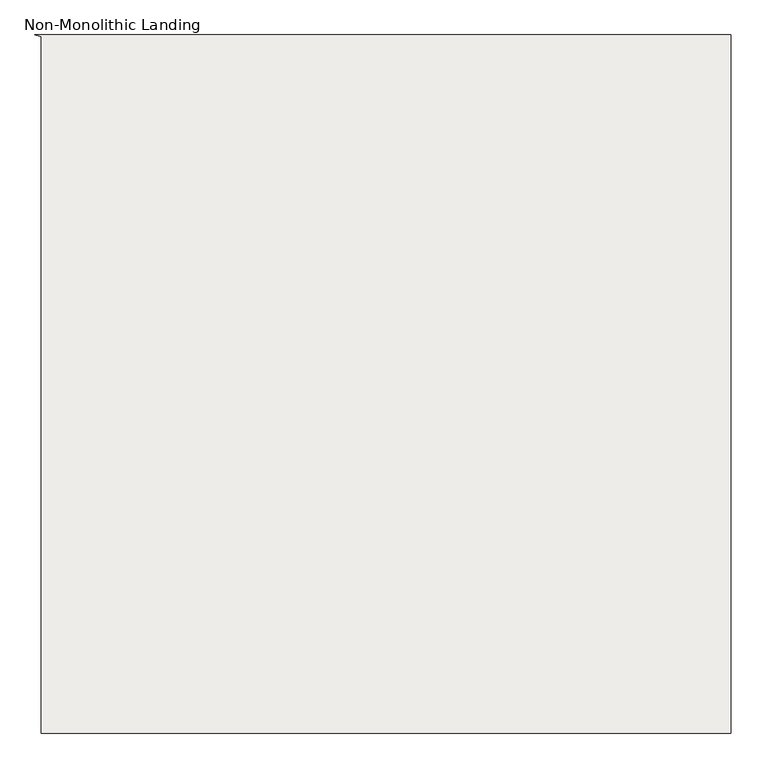
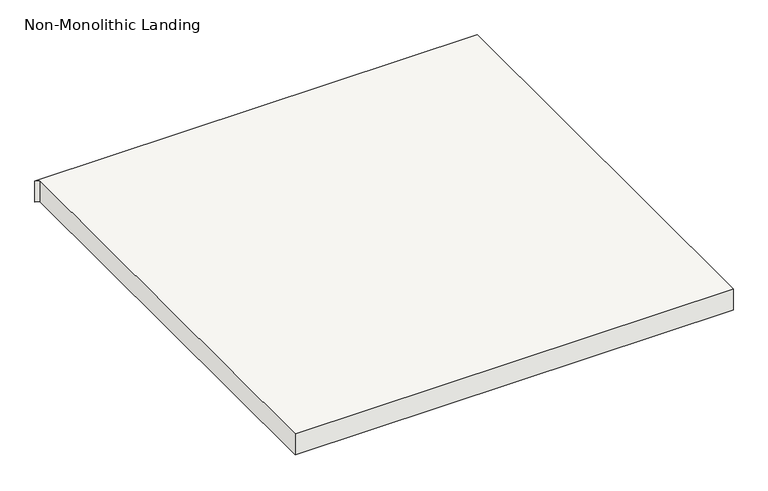
"""IFC4 building model written with IfcOpenShell, lengths in millimetres: slab geometry, Non-Monolithic Landing."""

from ifc_helpers import new_model, si_unit, frame, origin, place, context, project, spatial, polyline, outline, extrude, source, transform, mapped, element, save


def non_monolithic_landing_3909d1ad(model_context):
    return source(origin(), model_context, "Body", "SweptSolid", [
        extrude(outline(polyline([(-9477.5794909, -3248.5618509), (-9477.5794909, -4251.1618509), (-10468.1794909, -4251.1618509), (-10468.1794909, -3251.1360696), (-10477.6052721, -3248.5618509), (-9477.5794909, -3248.5618509)])), frame((0.0, 0.0, 8421.6470588), z_axis=(0.0, 0.0, 1.0), x_axis=(1.0, 0.0, 0.0)), (0.0, 0.0, 1.0), 50.0),
    ])


if __name__ == "__main__":
    model = new_model("IFC4")
    model_context = context("Model", 3, world=origin())
    ifc_project = project(units=[si_unit("LENGTHUNIT", "METRE", prefix="MILLI")], contexts=[model_context])
    site = spatial("IfcSite", under=ifc_project)
    building = spatial("IfcBuilding", under=site)
    placement = place(None, origin())
    non_monolithic_landing_shape = non_monolithic_landing_3909d1ad(model_context)
    element("IfcSlab", 1, ObjectType="Non-Monolithic Landing", at=placement, inside=building, context=model_context, shape_type="MappedRepresentation", body=[
        mapped(non_monolithic_landing_shape, transform((0.0, 0.0, 0.0), x_axis=(1.0, 0.0, 0.0), y_axis=(0.0, 1.0, 0.0), z_axis=(0.0, 0.0, 1.0))),
    ])
    save(model, "model.ifc")
